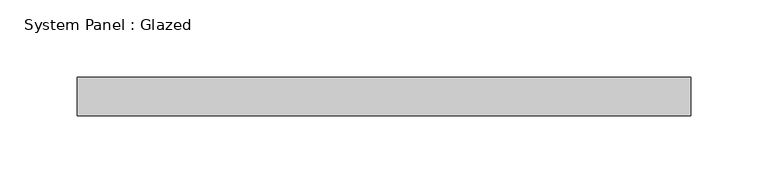
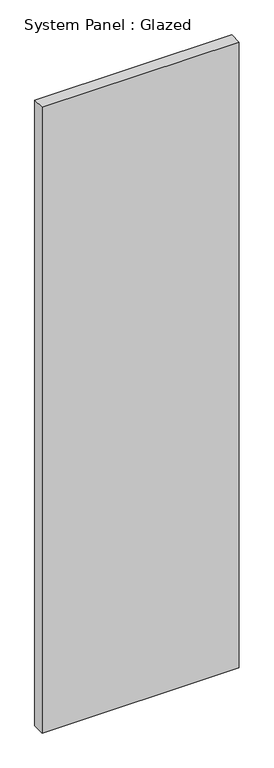
"""IFC4 building model written with IfcOpenShell, lengths in millimetres: plate geometry, System Panel : Glazed."""

from ifc_helpers import new_model, si_unit, origin, origin_with_axes, place, context, project, spatial, polyline, outline, extrude, source, transform, mapped, element, save


def system_panel_glazed_e520f566(model_context):
    return source(origin(), model_context, "Body", "SweptSolid", [
        extrude(outline(polyline([(198.4375, 24.5), (-198.4375, 24.5), (-198.4375, 49.5), (198.4375, 49.5), (198.4375, 24.5)])), origin_with_axes(), (0.0, 0.0, 1.0), 1330.8429687),
    ])


if __name__ == "__main__":
    model = new_model("IFC4")
    model_context = context("Model", 3, world=origin())
    ifc_project = project(units=[si_unit("LENGTHUNIT", "METRE", prefix="MILLI")], contexts=[model_context])
    site = spatial("IfcSite", under=ifc_project)
    building = spatial("IfcBuilding", under=site)
    placement = place(None, origin())
    system_panel_glazed_shape = system_panel_glazed_e520f566(model_context)
    element("IfcPlate", 1, ObjectType="System Panel : Glazed", at=placement, inside=building, context=model_context, shape_type="MappedRepresentation", body=[
        mapped(system_panel_glazed_shape, transform((0.0, 0.0, 0.0), x_axis=(1.0, 0.0, 0.0), y_axis=(0.0, 1.0, 0.0), z_axis=(0.0, 0.0, 1.0))),
    ])
    save(model, "model.ifc")

# Revit data of these elements
# Type "System Panel : Glazed"
#   Keynote = "H11"
#   Construction Type Id = "GSP4R"
#   Analytic Construction = "1/8 in Pilkington single glazing"
#   Visual Light Transmittance = 0.9
#   Solar Heat Gain Coefficient = 0.86
#   Heat Transfer Coefficient (U) = 6.7069 W/(m²·K)
#   Define Thermal Properties by = 1
# Element 1 (IfcPlate, "System Panel : Glazed")
#   Materials on its faces: "Glass"
# Materials
#   "Glass": class "Glass", colour RGB 0 128 192, transparency 0.9, Description = "Soda Lime Glass", Cost = 0
